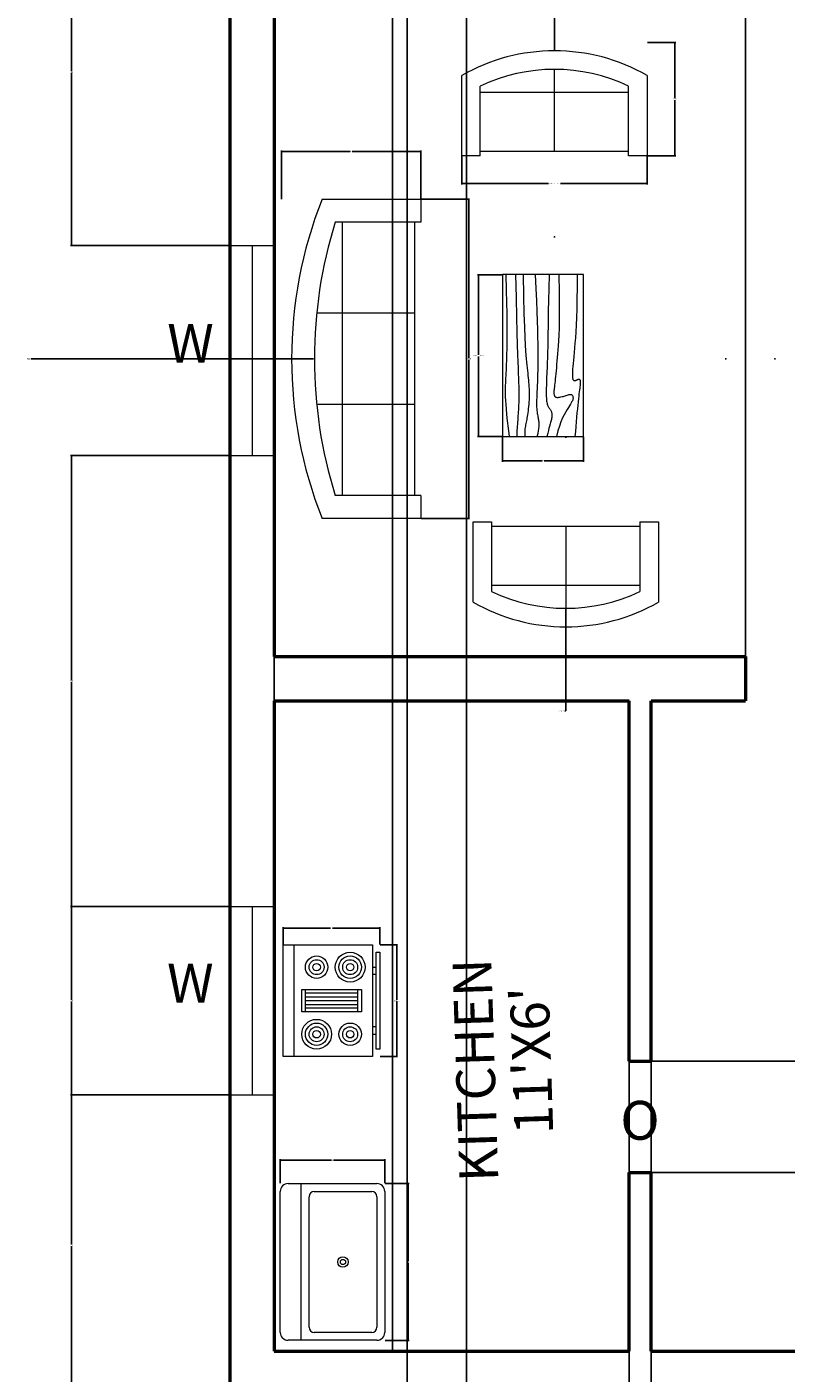
# Model space of a CAD drawing. Units: feet. Extents: x 1657 to 2001, y 1678 to 2367.
# Tile 2 of 4: x 1657 to 1811, y 1847 to 2120. Entities that reach past the tile are written whole.
import ezdxf

# ---------------------------------------------------------------- set-up
doc = ezdxf.new("R2010")
doc.units = ezdxf.units.FT
for name, color, linetype, lineweight in [('A-ANNO-DIMS', 2, 'Continuous', 18), ('A-ANNO-TEXT', 7, 'Continuous', 18), ('A-AREA-IDEN', 7, 'Continuous', 25), ('A-EQPM', 9, 'Continuous', 18), ('A-FLOR-CASE', 8, 'Continuous', 25), ('A-FLOR-FIXT', 8, 'Continuous', 18), ('A-FURN', 8, 'Continuous', 18), ('A-GLAZ', 4, 'Continuous', 18), ('A-WALL', 7, 'Continuous', 50)]:
    doc.layers.add(name, color=color, linetype=linetype, lineweight=lineweight)
doc.styles.get("Standard").update_dxf_attribs({"font": 'arial.ttf'})
doc.dimstyles.get("Standard").update_dxf_attribs({"dimtxt": 0.18, "dimasz": 0.18, "dimexe": 0.18, "dimexo": 0.0625, "dimgap": 0.09, "dimtad": 0, "dimtih": 1, "dimtoh": 1, "dimdec": 4, "dimzin": 0, "dimdsep": 46, "dimtxsty": 'Standard', "dimcen": 0.09, "dimadec": 0, "dimazin": 0, "dimtfac": 1, "dimtdec": 4, "dimtofl": 0, "dimtmove": 0, "dimatfit": 3, "dimfxl": 1, "dimtolj": 1, "dimtzin": 0, "dimarcsym": 0})

# ---------------------------------------------------------------- blocks, each defined once
blk = doc.blocks.new('Sofa - Roundback 7 ft.')
for p, q in [((-12.00002, -32.4421), (-12.00003, -6.5971)), ((11.99997, -32.4421), (11.99998, -6.5971)), ((-36.000027, -34), (-36.000027, -11.4696)), ((-35.999844, -13.3819), (35.9998, -13.3819)), ((35.99998, -34), (35.99998, -11.4696)), ((-36.000027, -32.4421), (35.99998, -32.4421))]:
    blk.add_line(p, q)
for points in [[(-36.000027, -34), (-42.000027, -34), (-42.000027, -8)], [(41.99998, -8), (41.99998, -34), (35.99998, -34)]]:
    blk.add_lwpolyline(points)
for centre, radius, start, end in [((0, -114.25), 114.25, 68.43141, 111.5686), ((-0.00001, -127.1968), 121.1968, 72.72033, 107.2797)]:
    blk.add_arc(centre, radius, start, end)
blk = doc.blocks.new('Sofa - Roundback Loveseat 5 ft.')
for p, q in [((0, -32.44198), (0, -5.99998)), ((-24, -33.99998), (-24, -11.46958)), ((24.00004, -33.99998), (24.00004, -11.46958)), ((-23.9998, -13.38178), (23.99986, -13.38178)), ((-24, -32.44198), (24.00004, -32.44198))]:
    blk.add_line(p, q)
for points in [[(-24, -33.99998), (-30, -33.99998), (-30, -7.99998)], [(30.00004, -7.99998), (30.00004, -33.99998), (24.00004, -33.99998)]]:
    blk.add_lwpolyline(points)
for centre, radius, start, end in [((0, -60.24998), 60.24998, 60.13715, 119.8628), ((0, -61.38438), 55.38444, 64.32083, 115.6792)]:
    blk.add_arc(centre, radius, start, end)
blk = doc.blocks.new('Table - Rectangular Woodgrain 60 x 30 in.')
for p, q in [((0, 0), (0, -30)), ((60, 0), (0, 0)), ((60, -30), (60, 0)), ((0, -30), (60, -30))]:
    blk.add_line(p, q)
for points in [[(0, -2.4), (4.8155, -2.418), (9.0302, -2.4688), (12.709, -2.5477), (15.9167, -2.65), (18.7181, -2.7711), (21.1781, -2.9063), (23.3616, -3.0508), (25.3333, -3.2), (27.1477, -3.3495), (28.8172, -3.4958), (30.3437, -3.636), (31.7291, -3.7667), (32.9756, -3.8849), (34.0849, -3.9875), (35.059, -4.0714), (35.9, -4.1334), (36.6114, -4.1711), (37.2041, -4.1854), (37.6906, -4.1779), (38.0833, -4.15), (38.3948, -4.1034), (38.6375, -4.0396), (38.8239, -3.9602), (38.9666, -3.8667), (39.0764, -3.7608), (39.1573, -3.6448), (39.2116, -3.521), (39.2416, -3.3917), (39.2498, -3.2593), (39.2385, -3.1261), (39.21, -2.9944), (39.1666, -2.8667), (39.111, -2.7447), (39.0468, -2.6281), (38.978, -2.5163), (38.9083, -2.4083), (38.8418, -2.3035), (38.7823, -2.201), (38.7337, -2.1001), (38.7, -2), (38.6844, -1.9003), (38.6875, -1.8021), (38.7094, -1.707), (38.75, -1.6167), (38.8094, -1.5326), (38.8875, -1.4563), (38.9844, -1.3893), (39.1, -1.3333), (39.2351, -1.2896), (39.3937, -1.2583), (39.5804, -1.2396), (39.8, -1.2333), (40.057, -1.2396), (40.3562, -1.2583), (40.7023, -1.2896), (41.1, -1.3333), (41.5547, -1.3895), (42.0755, -1.4573), (42.6721, -1.5361), (43.3542, -1.625), (44.1316, -1.7233), (45.014, -1.8302), (46.0114, -1.9449), (47.1333, -2.0667), (48.3862, -2.1947), (49.7625, -2.3281), (51.2513, -2.4663), (52.8416, -2.6083), (54.5226, -2.7535), (56.2833, -2.9011), (58.1127, -3.0501), (60, -3.2)], [(0, -9.2), (6.5759, -9.0858), (11.9385, -9.0365), (16.2527, -9.0418), (19.6833, -9.0917), (22.3952, -9.1759), (24.5531, -9.2844), (26.322, -9.4069), (27.8666, -9.5333), (29.3241, -9.6553), (30.7203, -9.7719), (32.0532, -9.8837), (33.3208, -9.9917), (34.5213, -10.0965), (35.6526, -10.199), (36.7128, -10.2999), (37.7, -10.4), (38.6129, -10.4996), (39.4531, -10.5969), (40.223, -10.6895), (40.925, -10.775), (41.5613, -10.8512), (42.1344, -10.9156), (42.6465, -10.966), (43.1, -11), (43.4976, -11.0158), (43.8437, -11.0136), (44.143, -10.9942), (44.4, -10.9583), (44.6195, -10.9069), (44.8062, -10.8406), (44.9648, -10.7603), (45.1, -10.6667), (45.2155, -10.5598), (45.3114, -10.4365), (45.3871, -10.2929), (45.4416, -10.125), (45.4743, -9.929), (45.4844, -9.7011), (45.4709, -9.4371), (45.4333, -9.1333), (45.3716, -8.7883), (45.2896, -8.4104), (45.1919, -8.0107), (45.0833, -7.6), (44.9685, -7.1893), (44.8521, -6.7896), (44.7388, -6.4117), (44.6333, -6.0667), (44.54, -5.7628), (44.4614, -5.4979), (44.4001, -5.2675), (44.3583, -5.0667), (44.3384, -4.8909), (44.3427, -4.7354), (44.3736, -4.5956), (44.4333, -4.4667), (44.5236, -4.3453), (44.6427, -4.2333), (44.7884, -4.1339), (44.9583, -4.05), (45.1501, -3.9849), (45.3614, -3.9417), (45.59, -3.9234), (45.8333, -3.9333), (46.0915, -3.9749), (46.3734, -4.0531), (46.6906, -4.1736), (47.0542, -4.3417), (47.4756, -4.5629), (47.9661, -4.8427), (48.5372, -5.1866), (49.2, -5.6), (49.9676, -6.0844), (50.8594, -6.625), (51.8965, -7.2031), (53.1, -7.8), (54.491, -8.3969), (56.0906, -8.975), (57.9199, -9.5156), (60, -10)], [(0, -12.8), (5.1847, -12.9322), (9.6213, -13.0323), (13.3963, -13.1059), (16.5958, -13.1583), (19.3063, -13.1952), (21.614, -13.2219), (23.6054, -13.2439), (25.3666, -13.2667), (26.9728, -13.2947), (28.4531, -13.3281), (29.8256, -13.3663), (31.1083, -13.4083), (32.3191, -13.4535), (33.476, -13.501), (34.597, -13.5501), (35.7, -13.6), (36.7984, -13.6497), (37.8875, -13.6979), (38.9578, -13.743), (40, -13.7833), (41.0047, -13.8174), (41.9625, -13.8438), (42.864, -13.8607), (43.7, -13.8667), (44.4631, -13.8604), (45.1552, -13.8417), (45.7801, -13.8104), (46.3416, -13.7667), (46.8439, -13.7104), (47.2906, -13.6417), (47.6858, -13.5604), (48.0333, -13.4667), (48.3375, -13.3608), (48.6042, -13.2448), (48.8396, -13.121), (49.05, -12.9917), (49.2417, -12.8593), (49.4208, -12.7261), (49.5937, -12.5944), (49.7667, -12.4667), (49.9452, -12.3451), (50.1323, -12.2313), (50.3303, -12.1268), (50.5416, -12.0333), (50.7686, -11.9524), (51.0135, -11.8854), (51.2788, -11.8341), (51.5666, -11.8), (51.8785, -11.7843), (52.2116, -11.7865), (52.562, -11.8059), (52.926, -11.8417), (53.2998, -11.8931), (53.6795, -11.9594), (54.0614, -12.0397), (54.4416, -12.1333), (54.8223, -12.2401), (55.2293, -12.3625), (55.6942, -12.5037), (56.2489, -12.6667), (56.9251, -12.8547), (57.7545, -13.0708), (58.7689, -13.3182), (60, -13.6)], [(0, -18), (5.124, -17.7273), (9.6609, -17.5057), (13.6705, -17.3303), (17.2125, -17.1958), (20.3467, -17.0973), (23.1328, -17.0297), (25.6307, -16.9878), (27.9, -16.9667), (29.9928, -16.9617), (31.9302, -16.9703), (33.7254, -16.9907), (35.3917, -17.0208), (36.9423, -17.0588), (38.3906, -17.1026), (39.7499, -17.1503), (41.0333, -17.2), (42.2519, -17.2496), (43.4073, -17.2969), (44.4986, -17.3395), (45.525, -17.375), (46.4858, -17.4012), (47.3802, -17.4156), (48.2074, -17.416), (48.9667, -17.4), (49.6583, -17.3662), (50.2872, -17.3167), (50.8595, -17.2547), (51.3812, -17.1833), (51.8584, -17.1057), (52.2971, -17.025), (52.7034, -16.9443), (53.0833, -16.8667), (53.443, -16.7951), (53.789, -16.7313), (54.128, -16.6768), (54.4666, -16.6334), (54.8115, -16.6024), (55.1693, -16.5854), (55.5465, -16.5841), (55.95, -16.6), (56.3828, -16.6337), (56.8346, -16.6823), (57.2915, -16.7418), (57.7396, -16.8084), (58.165, -16.878), (58.5539, -16.9469), (58.8924, -17.0111), (59.1666, -17.0667), (59.3679, -17.1107), (59.5078, -17.1438), (59.6032, -17.1675), (59.6708, -17.1833), (59.7275, -17.193), (59.7901, -17.1979), (59.8753, -17.1998), (60, -17.2)], [(0, -22.4), (8.0098, -22.2501), (14.4094, -22.1011), (19.4168, -21.9535), (23.25, -21.8083), (26.1269, -21.6663), (28.2656, -21.5281), (29.884, -21.3947), (31.2, -21.2667), (32.3967, -21.1448), (33.5172, -21.0292), (34.5697, -20.9198), (35.5625, -20.8167), (36.5037, -20.7198), (37.4015, -20.6292), (38.2642, -20.5448), (39.1, -20.4667), (39.9164, -20.3951), (40.7187, -20.3313), (41.5117, -20.2768), (42.3, -20.2333), (43.0883, -20.2024), (43.8812, -20.1854), (44.6836, -20.1841), (45.5, -20.2), (46.3328, -20.234), (47.1747, -20.2844), (48.0163, -20.3488), (48.8479, -20.425), (49.66, -20.5106), (50.4429, -20.6031), (51.1872, -20.7004), (51.8833, -20.8), (52.5246, -20.8999), (53.1166, -20.9995), (53.6681, -21.0983), (54.1875, -21.1958), (54.6834, -21.2919), (55.1646, -21.3859), (55.6394, -21.4777), (56.1167, -21.5667), (56.6028, -21.6515), (57.0961, -21.7266), (57.5929, -21.7852), (58.0896, -21.8208), (58.5823, -21.8268), (59.0674, -21.7964), (59.5412, -21.723), (60, -21.6)], [(0, -25.2), (8.6355, -25.0504), (15.7026, -24.9031), (21.4049, -24.7606), (25.9458, -24.625), (29.529, -24.4988), (32.3578, -24.3844), (34.6359, -24.284), (36.5667, -24.2), (38.3213, -24.1341), (39.9417, -24.0854), (41.437, -24.0523), (42.8167, -24.0333), (44.0901, -24.0268), (45.2667, -24.0313), (46.3557, -24.0451), (47.3667, -24.0667), (48.309, -24.0947), (49.1928, -24.1287), (50.0284, -24.168), (50.826, -24.2125), (51.5959, -24.2617), (52.3483, -24.3151), (53.0935, -24.3725), (53.8417, -24.4334), (54.6009, -24.497), (55.3699, -24.561), (56.1454, -24.6226), (56.9239, -24.6792), (57.7021, -24.7279), (58.4764, -24.7662), (59.2435, -24.7911), (60, -24.8)], [(0, -28.8), (5.6867, -28.6681), (10.45, -28.5698), (14.407, -28.5012), (17.675, -28.4584), (20.3711, -28.4374), (22.6125, -28.4344), (24.5164, -28.4455), (26.2, -28.4667), (27.762, -28.4947), (29.2276, -28.5281), (30.6033, -28.5663), (31.8958, -28.6084), (33.1118, -28.6535), (34.2578, -28.7011), (35.3405, -28.7501), (36.3666, -28.8), (37.3443, -28.8497), (38.288, -28.8974), (39.2137, -28.9412), (40.1375, -28.9792), (41.0753, -29.0093), (42.0432, -29.0297), (43.0572, -29.0384), (44.1333, -29.0333), (45.2936, -29.0114), (46.5843, -28.9641), (48.0579, -28.8816), (49.7666, -28.7542), (51.7629, -28.5721), (54.0989, -28.3255), (56.8272, -28.0048), (60, -27.6)]]:
    blk.add_lwpolyline(points)
blk = doc.blocks.new('Range-Oven - 30 in top')
for p, q in [((0, -3), (30, -3)), ((12, -6), (18, -6)), ((13, -20), (13, -6)), ((14, -6), (14, -20)), ((15, -20), (15, -6)), ((16, -6), (16, -20)), ((17, -20), (17, -6)), ((18, -20), (12, -20)), ((6, -24), (6, -25)), ((8, -25), (8, -24)), ((22, -25), (22, -24)), ((24, -24), (24, -25))]:
    blk.add_line(p, q)
for points in [[(0, -24), (0, 0), (30, 0), (30, -24)], [(12, -21), (12, -5), (18, -5), (18, -21)], [(2, -26), (2, -25), (28, -25), (28, -26)]]:
    blk.add_lwpolyline(points, close=True)
for centre, radius in [((6, -9), 4), ((6, -9), 3), ((6, -9), 2), ((24, -9), 3), ((24, -9), 2), ((6, -9), 1), ((24, -9), 1), ((24, -18), 4), ((6, -18), 3), ((6, -18), 2), ((6, -18), 1), ((24, -18), 3), ((24, -18), 2), ((24, -18), 1)]:
    blk.add_circle(centre, radius)
blk = doc.blocks.new('Sink-single - 30 in top')
blk.add_line((-15, -3.999996), (15, -3.999996))
for points in [[(-13.5, 0), (13.5, 0)], [(-15, -18.499996), (-15, -1.5)], [(15, -1.5), (15, -18.499996)], [(-13.5, -17.499996), (-13.5, -6.499996)], [(-12.5, -5.499996), (12.5, -5.499996)], [(13.5, -6.499996), (13.5, -17.499996)], [(13.5, -19.999996), (-13.5, -19.999996)], [(12.5, -18.499996), (-12.5, -18.499996)]]:
    blk.add_lwpolyline(points)
for radius in [1, 0.5]:
    blk.add_circle((0, -11.999996), radius)
for centre, radius, start, end in [((-13.5, -1.5), 1.5, 90, 180), ((13.5, -1.5), 1.5, 0, 90), ((-12.5, -6.499996), 1, 90, 180), ((12.5, -6.499996), 1, 0, 90), ((-12.5, -17.499996), 1, 180, 270), ((12.5, -17.499996), 1, 270, 0), ((-13.5, -18.499996), 1.5, 180, 270), ((13.5, -18.499996), 1.5, 270, 0)]:
    blk.add_arc(centre, radius, start, end)
blk = doc.blocks.new('WIN-HALL')
for p, q in [((0, 42.59), (9, 42.59)), ((4.5, 42.59), (4.5, 0)), ((0, 0), (9, 0))]:
    blk.add_line(p, q)
blk = doc.blocks.new('*D16')
at = {"layer": 'A-ANNO-DIMS', "color": 0, "lineweight": -2, "transparency": 16777216}
for p, q in [((1745.34, 2093.87), (1745.34, 2088.11)), ((1782.96, 2093.87), (1782.96, 2088.11)), ((1745.52, 2088.29), (1762.93, 2088.29)), ((1782.78, 2088.29), (1765.37, 2088.29))]:
    blk.add_line(p, q, dxfattribs=at)
at = {"layer": 'A-ANNO-DIMS', "color": 0, "transparency": 16777216}
for points in [[(1745.52, 2088.32), (1745.52, 2088.26), (1745.34, 2088.29)], [(1782.78, 2088.32), (1782.78, 2088.26), (1782.96, 2088.29)]]:
    blk.add_solid(points, dxfattribs=at)
at = {"layer": 'Defpoints', "color": 0, "transparency": 16777216}
for p in [(1745.34, 2093.93), (1782.96, 2093.93), (1782.96, 2088.29)]:
    blk.add_point(p, dxfattribs=at)
at = {"layer": 'A-ANNO-DIMS', "color": 0, "transparency": 16777216, "insert": (1764.15, 2088.29), "char_height": 0.18, "attachment_point": 5}
blk.add_mtext('\\A1;LOVESEAT 38 TYP.', dxfattribs=at)
blk = doc.blocks.new('*D17')
at = {"layer": 'A-ANNO-DIMS', "color": 0, "lineweight": -2, "transparency": 16777216}
for p, q in [((1783.02, 2116.92), (1788.78, 2116.92)), ((1788.6, 2116.74), (1788.6, 2105.61)), ((1788.6, 2094.11), (1788.6, 2105.24)), ((1783.02, 2093.93), (1788.78, 2093.93))]:
    blk.add_line(p, q, dxfattribs=at)
at = {"layer": 'A-ANNO-DIMS', "color": 0, "transparency": 16777216}
for points in [[(1788.57, 2116.74), (1788.63, 2116.74), (1788.6, 2116.92)], [(1788.57, 2094.11), (1788.63, 2094.11), (1788.6, 2093.93)]]:
    blk.add_solid(points, dxfattribs=at)
at = {"layer": 'Defpoints', "color": 0, "transparency": 16777216}
for p in [(1782.96, 2116.92), (1788.6, 2116.92), (1782.96, 2093.93)]:
    blk.add_point(p, dxfattribs=at)
at = {"layer": 'A-ANNO-DIMS', "color": 0, "transparency": 16777216, "insert": (1788.6, 2105.42), "char_height": 0.18, "attachment_point": 5}
blk.add_mtext('\\A1;23 TYP.', dxfattribs=at)
blk = doc.blocks.new('*D18')
at = {"layer": 'A-ANNO-DIMS', "color": 0, "lineweight": -2, "transparency": 16777216}
for p, q in [((1737.09, 2085.11), (1746.92, 2085.11)), ((1746.74, 2084.93), (1746.74, 2052.91)), ((1746.74, 2020.53), (1746.74, 2052.55)), ((1737.09, 2020.35), (1746.92, 2020.35))]:
    blk.add_line(p, q, dxfattribs=at)
at = {"layer": 'A-ANNO-DIMS', "color": 0, "transparency": 16777216}
for points in [[(1746.71, 2084.93), (1746.77, 2084.93), (1746.74, 2085.11)], [(1746.71, 2020.53), (1746.77, 2020.53), (1746.74, 2020.35)]]:
    blk.add_solid(points, dxfattribs=at)
at = {"layer": 'Defpoints', "color": 0, "transparency": 16777216}
for p in [(1737.03, 2085.11), (1746.74, 2085.11), (1737.03, 2020.35)]:
    blk.add_point(p, dxfattribs=at)
at = {"layer": 'A-ANNO-DIMS', "color": 0, "transparency": 16777216, "insert": (1746.74, 2052.73), "char_height": 0.18, "attachment_point": 5}
blk.add_mtext('\\A1;SOFA 65', dxfattribs=at)
blk = doc.blocks.new('*D19')
at = {"layer": 'A-ANNO-DIMS', "color": 0, "lineweight": -2, "transparency": 16777216}
for p, q in [((1708.76, 2085.17), (1708.76, 2095.01)), ((1708.94, 2094.83), (1722.67, 2094.83)), ((1736.85, 2094.83), (1723.11, 2094.83)), ((1737.03, 2085.17), (1737.03, 2095.01))]:
    blk.add_line(p, q, dxfattribs=at)
at = {"layer": 'A-ANNO-DIMS', "color": 0, "transparency": 16777216}
for points in [[(1708.94, 2094.86), (1708.94, 2094.8), (1708.76, 2094.83)], [(1736.85, 2094.86), (1736.85, 2094.8), (1737.03, 2094.83)]]:
    blk.add_solid(points, dxfattribs=at)
at = {"layer": 'Defpoints', "color": 0, "transparency": 16777216}
for p in [(1708.76, 2094.83), (1708.76, 2085.11), (1737.03, 2085.11)]:
    blk.add_point(p, dxfattribs=at)
at = {"layer": 'A-ANNO-DIMS', "color": 0, "transparency": 16777216, "insert": (1722.89, 2094.83), "char_height": 0.18, "attachment_point": 5}
blk.add_mtext('\\A1;28', dxfattribs=at)
blk = doc.blocks.new('*D20')
at = {"layer": 'A-ANNO-DIMS', "color": 0, "lineweight": -2, "transparency": 16777216}
for p, q in [((1753.57, 2069.81), (1748.52, 2069.81)), ((1748.7, 2069.63), (1748.7, 2053.56)), ((1748.7, 2037.13), (1748.7, 2053.2)), ((1753.57, 2036.95), (1748.52, 2036.95))]:
    blk.add_line(p, q, dxfattribs=at)
at = {"layer": 'A-ANNO-DIMS', "color": 0, "transparency": 16777216}
for points in [[(1748.67, 2069.63), (1748.73, 2069.63), (1748.7, 2069.81)], [(1748.67, 2037.13), (1748.73, 2037.13), (1748.7, 2036.95)]]:
    blk.add_solid(points, dxfattribs=at)
at = {"layer": 'Defpoints', "color": 0, "transparency": 16777216}
for p in [(1753.63, 2069.81), (1748.7, 2036.95), (1753.63, 2036.95)]:
    blk.add_point(p, dxfattribs=at)
at = {"layer": 'A-ANNO-DIMS', "color": 0, "transparency": 16777216, "insert": (1748.7, 2053.38), "char_height": 0.18, "attachment_point": 5}
blk.add_mtext('\\A1;COFFEE TABLE 33', dxfattribs=at)
blk = doc.blocks.new('*D21')
at = {"layer": 'A-ANNO-DIMS', "color": 0, "lineweight": -2, "transparency": 16777216}
for p, q in [((1753.63, 2036.88), (1753.63, 2031.84)), ((1770.07, 2036.88), (1770.07, 2031.84)), ((1753.81, 2032.02), (1761.64, 2032.02)), ((1769.89, 2032.02), (1762.06, 2032.02))]:
    blk.add_line(p, q, dxfattribs=at)
at = {"layer": 'A-ANNO-DIMS', "color": 0, "transparency": 16777216}
for points in [[(1753.81, 2032.05), (1753.81, 2031.99), (1753.63, 2032.02)], [(1769.89, 2032.05), (1769.89, 2031.99), (1770.07, 2032.02)]]:
    blk.add_solid(points, dxfattribs=at)
at = {"layer": 'Defpoints', "color": 0, "transparency": 16777216}
for p in [(1753.63, 2036.95), (1770.07, 2036.95), (1770.07, 2032.02)]:
    blk.add_point(p, dxfattribs=at)
at = {"layer": 'A-ANNO-DIMS', "color": 0, "transparency": 16777216, "insert": (1761.85, 2032.02), "char_height": 0.18, "attachment_point": 5}
blk.add_mtext('\\A1;16', dxfattribs=at)
blk = doc.blocks.new('*D24')
at = {"layer": 'A-ANNO-DIMS', "color": 0, "lineweight": -2, "transparency": 16777216}
for p, q in [((1728.8, 1933.8), (1732.33, 1933.8)), ((1732.15, 1933.62), (1732.15, 1922.64)), ((1732.15, 1911.29), (1732.15, 1922.27)), ((1728.8, 1911.11), (1732.33, 1911.11))]:
    blk.add_line(p, q, dxfattribs=at)
at = {"layer": 'A-ANNO-DIMS', "color": 0, "transparency": 16777216}
for points in [[(1732.12, 1933.62), (1732.18, 1933.62), (1732.15, 1933.8)], [(1732.12, 1911.29), (1732.18, 1911.29), (1732.15, 1911.11)]]:
    blk.add_solid(points, dxfattribs=at)
at = {"layer": 'Defpoints', "color": 0, "transparency": 16777216}
for p in [(1728.74, 1933.8), (1732.15, 1933.8), (1728.74, 1911.11)]:
    blk.add_point(p, dxfattribs=at)
at = {"layer": 'A-ANNO-DIMS', "color": 0, "transparency": 16777216, "insert": (1732.15, 1922.45), "char_height": 0.18, "attachment_point": 5}
blk.add_mtext('\\A1;RANGE 23', dxfattribs=at)
blk = doc.blocks.new('*D25')
at = {"layer": 'A-ANNO-DIMS', "color": 0, "lineweight": -2, "transparency": 16777216}
for p, q in [((1709.07, 1933.86), (1709.07, 1937.38)), ((1709.25, 1937.2), (1718.69, 1937.2)), ((1728.56, 1937.2), (1719.13, 1937.2)), ((1728.74, 1933.86), (1728.74, 1937.38))]:
    blk.add_line(p, q, dxfattribs=at)
at = {"layer": 'A-ANNO-DIMS', "color": 0, "transparency": 16777216}
for points in [[(1709.25, 1937.23), (1709.25, 1937.17), (1709.07, 1937.2)], [(1728.56, 1937.23), (1728.56, 1937.17), (1728.74, 1937.2)]]:
    blk.add_solid(points, dxfattribs=at)
at = {"layer": 'Defpoints', "color": 0, "transparency": 16777216}
for p in [(1709.07, 1937.2), (1709.07, 1933.8), (1728.74, 1933.8)]:
    blk.add_point(p, dxfattribs=at)
at = {"layer": 'A-ANNO-DIMS', "color": 0, "transparency": 16777216, "insert": (1718.91, 1937.2), "char_height": 0.18, "attachment_point": 5}
blk.add_mtext('\\A1;20', dxfattribs=at)
blk = doc.blocks.new('*D26')
at = {"layer": 'A-ANNO-DIMS', "color": 0, "lineweight": -2, "transparency": 16777216}
for p, q in [((1729.77, 1885.33), (1734.66, 1885.33)), ((1734.48, 1885.15), (1734.48, 1869.61)), ((1734.48, 1853.7), (1734.48, 1869.24)), ((1729.77, 1853.52), (1734.66, 1853.52))]:
    blk.add_line(p, q, dxfattribs=at)
at = {"layer": 'A-ANNO-DIMS', "color": 0, "transparency": 16777216}
for points in [[(1734.45, 1885.15), (1734.51, 1885.15), (1734.48, 1885.33)], [(1734.45, 1853.7), (1734.51, 1853.7), (1734.48, 1853.52)]]:
    blk.add_solid(points, dxfattribs=at)
at = {"layer": 'Defpoints', "color": 0, "transparency": 16777216}
for p in [(1729.71, 1885.33), (1734.48, 1885.33), (1729.71, 1853.52)]:
    blk.add_point(p, dxfattribs=at)
at = {"layer": 'A-ANNO-DIMS', "color": 0, "transparency": 16777216, "insert": (1734.48, 1869.42), "char_height": 0.18, "attachment_point": 5}
blk.add_mtext('\\A1;SINK 32', dxfattribs=at)
blk = doc.blocks.new('*D27')
at = {"layer": 'A-ANNO-DIMS', "color": 0, "lineweight": -2, "transparency": 16777216}
for p, q in [((1708.51, 1885.39), (1708.51, 1890.28)), ((1708.69, 1890.1), (1718.91, 1890.1)), ((1729.53, 1890.1), (1719.31, 1890.1)), ((1729.71, 1885.39), (1729.71, 1890.28))]:
    blk.add_line(p, q, dxfattribs=at)
at = {"layer": 'A-ANNO-DIMS', "color": 0, "transparency": 16777216}
for points in [[(1708.69, 1890.13), (1708.69, 1890.07), (1708.51, 1890.1)], [(1729.53, 1890.13), (1729.53, 1890.07), (1729.71, 1890.1)]]:
    blk.add_solid(points, dxfattribs=at)
at = {"layer": 'Defpoints', "color": 0, "transparency": 16777216}
for p in [(1708.51, 1890.1), (1708.51, 1885.33), (1729.71, 1885.33)]:
    blk.add_point(p, dxfattribs=at)
at = {"layer": 'A-ANNO-DIMS', "color": 0, "transparency": 16777216, "insert": (1719.11, 1890.1), "char_height": 0.18, "attachment_point": 5}
blk.add_mtext('\\A1;21', dxfattribs=at)
blk = doc.blocks.new('*D37')
at = {"layer": 'A-ANNO-DIMS', "color": 0, "lineweight": -2, "transparency": 16777216}
for p, q in [((1734.28, 1770.36), (1734.28, 2366.63)), ((1734.46, 2366.45), (1740.08, 2366.45)), ((1746.1, 2366.45), (1740.49, 2366.45)), ((1746.28, 1770.36), (1746.28, 2366.63))]:
    blk.add_line(p, q, dxfattribs=at)
at = {"layer": 'A-ANNO-DIMS', "color": 0, "transparency": 16777216}
for points in [[(1734.46, 2366.48), (1734.46, 2366.42), (1734.28, 2366.45)], [(1746.1, 2366.48), (1746.1, 2366.42), (1746.28, 2366.45)]]:
    blk.add_solid(points, dxfattribs=at)
at = {"layer": 'Defpoints', "color": 0, "transparency": 16777216}
for p in [(1746.28, 2366.45), (1734.28, 1770.3), (1746.28, 1770.3)]:
    blk.add_point(p, dxfattribs=at)
at = {"layer": 'A-ANNO-DIMS', "color": 0, "transparency": 16777216, "insert": (1740.28, 2366.45), "char_height": 0.18, "attachment_point": 5}
blk.add_mtext('\\A1;12', dxfattribs=at)
blk = doc.blocks.new('*D38')
at = {"layer": 'A-ANNO-DIMS', "color": 0, "lineweight": -2, "transparency": 16777216}
for p, q in [((1698.28, 1770.36), (1698.28, 2366.63)), ((1698.46, 2366.45), (1716.07, 2366.45)), ((1734.1, 2366.45), (1716.5, 2366.45)), ((1734.28, 1770.36), (1734.28, 2366.63))]:
    blk.add_line(p, q, dxfattribs=at)
at = {"layer": 'A-ANNO-DIMS', "color": 0, "transparency": 16777216}
for points in [[(1698.46, 2366.48), (1698.46, 2366.42), (1698.28, 2366.45)], [(1734.1, 2366.48), (1734.1, 2366.42), (1734.28, 2366.45)]]:
    blk.add_solid(points, dxfattribs=at)
at = {"layer": 'Defpoints', "color": 0, "transparency": 16777216}
for p in [(1734.28, 2366.45), (1698.28, 1770.3), (1734.28, 1770.3)]:
    blk.add_point(p, dxfattribs=at)
at = {"layer": 'A-ANNO-DIMS', "color": 0, "transparency": 16777216, "insert": (1716.28, 2366.45), "char_height": 0.18, "attachment_point": 5}
blk.add_mtext('\\A1;36', dxfattribs=at)
blk = doc.blocks.new('*D43')
at = {"layer": 'A-ANNO-DIMS', "color": 0, "lineweight": -2, "transparency": 16777216}
for p, q in [((1698.22, 1903.34), (1665.95, 1903.34)), ((1666.13, 1903.16), (1666.13, 1873)), ((1666.13, 1842.48), (1666.13, 1872.64)), ((1698.22, 1842.3), (1665.95, 1842.3))]:
    blk.add_line(p, q, dxfattribs=at)
at = {"layer": 'A-ANNO-DIMS', "color": 0, "transparency": 16777216}
for points in [[(1666.1, 1903.16), (1666.16, 1903.16), (1666.13, 1903.34)], [(1666.1, 1842.48), (1666.16, 1842.48), (1666.13, 1842.3)]]:
    blk.add_solid(points, dxfattribs=at)
at = {"layer": 'Defpoints', "color": 0, "transparency": 16777216}
for p in [(1666.13, 1903.34), (1698.28, 1903.34), (1698.28, 1842.3)]:
    blk.add_point(p, dxfattribs=at)
at = {"layer": 'A-ANNO-DIMS', "color": 0, "transparency": 16777216, "insert": (1666.13, 1872.82), "char_height": 0.18, "attachment_point": 5}
blk.add_mtext('\\A1;61.04', dxfattribs=at)
blk = doc.blocks.new('*D44')
at = {"layer": 'A-ANNO-DIMS', "color": 0, "lineweight": -2, "transparency": 16777216}
for p, q in [((1698.22, 1941.58), (1665.95, 1941.58)), ((1666.13, 1941.4), (1666.13, 1922.64)), ((1666.13, 1903.52), (1666.13, 1922.28)), ((1698.22, 1903.34), (1665.95, 1903.34))]:
    blk.add_line(p, q, dxfattribs=at)
at = {"layer": 'A-ANNO-DIMS', "color": 0, "transparency": 16777216}
for points in [[(1666.1, 1941.4), (1666.16, 1941.4), (1666.13, 1941.58)], [(1666.1, 1903.52), (1666.16, 1903.52), (1666.13, 1903.34)]]:
    blk.add_solid(points, dxfattribs=at)
at = {"layer": 'Defpoints', "color": 0, "transparency": 16777216}
for p in [(1666.13, 1941.58), (1698.28, 1941.58), (1698.28, 1903.34)]:
    blk.add_point(p, dxfattribs=at)
at = {"layer": 'A-ANNO-DIMS', "color": 0, "transparency": 16777216, "insert": (1666.13, 1922.46), "char_height": 0.18, "attachment_point": 5}
blk.add_mtext('\\A1;38.24', dxfattribs=at)
blk = doc.blocks.new('*D45')
at = {"layer": 'A-ANNO-DIMS', "color": 0, "lineweight": -2, "transparency": 16777216}
for p, q in [((1698.22, 2033.14), (1665.95, 2033.14)), ((1666.13, 2032.96), (1666.13, 1987.54)), ((1666.13, 1941.76), (1666.13, 1987.18)), ((1698.22, 1941.58), (1665.95, 1941.58))]:
    blk.add_line(p, q, dxfattribs=at)
at = {"layer": 'A-ANNO-DIMS', "color": 0, "transparency": 16777216}
for points in [[(1666.1, 2032.96), (1666.16, 2032.96), (1666.13, 2033.14)], [(1666.1, 1941.76), (1666.16, 1941.76), (1666.13, 1941.58)]]:
    blk.add_solid(points, dxfattribs=at)
at = {"layer": 'Defpoints', "color": 0, "transparency": 16777216}
for p in [(1666.13, 2033.14), (1698.28, 2033.14), (1698.28, 1941.58)]:
    blk.add_point(p, dxfattribs=at)
at = {"layer": 'A-ANNO-DIMS', "color": 0, "transparency": 16777216, "insert": (1666.13, 1987.36), "char_height": 0.18, "attachment_point": 5}
blk.add_mtext('\\A1;91.57', dxfattribs=at)
blk = doc.blocks.new('*D46')
at = {"layer": 'A-ANNO-DIMS', "color": 0, "lineweight": -2, "transparency": 16777216}
for p, q in [((1698.22, 2146.17), (1665.95, 2146.17)), ((1666.13, 2145.99), (1666.13, 2111.13)), ((1666.13, 2075.91), (1666.13, 2110.77)), ((1698.22, 2075.73), (1665.95, 2075.73))]:
    blk.add_line(p, q, dxfattribs=at)
at = {"layer": 'A-ANNO-DIMS', "color": 0, "transparency": 16777216}
for points in [[(1666.1, 2145.99), (1666.16, 2145.99), (1666.13, 2146.17)], [(1666.1, 2075.91), (1666.16, 2075.91), (1666.13, 2075.73)]]:
    blk.add_solid(points, dxfattribs=at)
at = {"layer": 'Defpoints', "color": 0, "transparency": 16777216}
for p in [(1666.13, 2146.17), (1698.28, 2146.17), (1698.28, 2075.73)]:
    blk.add_point(p, dxfattribs=at)
at = {"layer": 'A-ANNO-DIMS', "color": 0, "transparency": 16777216, "insert": (1666.13, 2110.95), "char_height": 0.18, "attachment_point": 5}
blk.add_mtext('\\A1;70.44', dxfattribs=at)
blk = doc.blocks.new('*D53')
at = {"layer": 'A-ANNO-DIMS', "color": 0, "lineweight": -2, "transparency": 16777216}
for p, q in [((1779.28, 1983.24), (1779.28, 1677.97)), ((1783.78, 1983.24), (1783.78, 1677.97)), ((1779.46, 1678.15), (1781.28, 1678.15)), ((1783.6, 1678.15), (1781.79, 1678.15))]:
    blk.add_line(p, q, dxfattribs=at)
at = {"layer": 'A-ANNO-DIMS', "color": 0, "transparency": 16777216}
for points in [[(1779.46, 1678.18), (1779.46, 1678.12), (1779.28, 1678.15)], [(1783.6, 1678.18), (1783.6, 1678.12), (1783.78, 1678.15)]]:
    blk.add_solid(points, dxfattribs=at)
at = {"layer": 'Defpoints', "color": 0, "transparency": 16777216}
for p in [(1779.28, 1983.3), (1783.78, 1983.3), (1783.78, 1678.15)]:
    blk.add_point(p, dxfattribs=at)
at = {"layer": 'A-ANNO-DIMS', "color": 0, "transparency": 16777216, "insert": (1781.53, 1678.15), "char_height": 0.18, "attachment_point": 5}
blk.add_mtext('\\A1;4.5', dxfattribs=at)
blk = doc.blocks.new('*D54')
at = {"layer": 'A-ANNO-DIMS', "color": 0, "lineweight": -2, "transparency": 16777216}
for p, q in [((1779.35, 1910.16), (2000.61, 1910.16)), ((2000.43, 1909.98), (2000.43, 1899.06)), ((2000.43, 1887.77), (2000.43, 1898.69)), ((1779.35, 1887.59), (2000.61, 1887.59))]:
    blk.add_line(p, q, dxfattribs=at)
at = {"layer": 'A-ANNO-DIMS', "color": 0, "transparency": 16777216}
for points in [[(2000.4, 1909.98), (2000.46, 1909.98), (2000.43, 1910.16)], [(2000.4, 1887.77), (2000.46, 1887.77), (2000.43, 1887.59)]]:
    blk.add_solid(points, dxfattribs=at)
at = {"layer": 'Defpoints', "color": 0, "transparency": 16777216}
for p in [(1779.28, 1910.16), (2000.43, 1910.16), (1779.28, 1887.59)]:
    blk.add_point(p, dxfattribs=at)
at = {"layer": 'A-ANNO-DIMS', "color": 0, "transparency": 16777216, "insert": (2000.43, 1898.88), "char_height": 0.18, "attachment_point": 5}
blk.add_mtext('\\A1;22.577', dxfattribs=at)
blk = doc.blocks.new('*D55')
at = {"layer": 'A-ANNO-DIMS', "color": 0, "lineweight": -2, "transparency": 16777216}
for p, q in [((1707.28, 1851.36), (1707.28, 2366.63)), ((1707.46, 2366.45), (1719.06, 2366.45)), ((1731.1, 2366.45), (1719.5, 2366.45)), ((1731.28, 1851.36), (1731.28, 2366.63))]:
    blk.add_line(p, q, dxfattribs=at)
at = {"layer": 'A-ANNO-DIMS', "color": 0, "transparency": 16777216}
for points in [[(1707.46, 2366.48), (1707.46, 2366.42), (1707.28, 2366.45)], [(1731.1, 2366.48), (1731.1, 2366.42), (1731.28, 2366.45)]]:
    blk.add_solid(points, dxfattribs=at)
at = {"layer": 'Defpoints', "color": 0, "transparency": 16777216}
for p in [(1731.28, 2366.45), (1707.28, 1851.3), (1731.28, 1851.3)]:
    blk.add_point(p, dxfattribs=at)
at = {"layer": 'A-ANNO-DIMS', "color": 0, "transparency": 16777216, "insert": (1719.28, 2366.45), "char_height": 0.18, "attachment_point": 5}
blk.add_mtext('\\A1;24', dxfattribs=at)
blk = doc.blocks.new('*D56')
at = {"layer": 'A-ANNO-DIMS', "color": 0, "lineweight": -2, "transparency": 16777216}
for p, q in [((1802.91, 1992.36), (1802.91, 2366.63)), ((1803.09, 2366.45), (1828.29, 2366.45)), ((1854.28, 2366.45), (1829.08, 2366.45)), ((1854.46, 1992.36), (1854.46, 2366.63))]:
    blk.add_line(p, q, dxfattribs=at)
at = {"layer": 'A-ANNO-DIMS', "color": 0, "transparency": 16777216}
for points in [[(1803.09, 2366.48), (1803.09, 2366.42), (1802.91, 2366.45)], [(1854.28, 2366.48), (1854.28, 2366.42), (1854.46, 2366.45)]]:
    blk.add_solid(points, dxfattribs=at)
at = {"layer": 'Defpoints', "color": 0, "transparency": 16777216}
for p in [(1854.46, 2366.45), (1802.91, 1992.3), (1854.46, 1992.3)]:
    blk.add_point(p, dxfattribs=at)
at = {"layer": 'A-ANNO-DIMS', "color": 0, "transparency": 16777216, "insert": (1828.68, 2366.45), "char_height": 0.18, "attachment_point": 5}
blk.add_mtext('\\A1;51.55', dxfattribs=at)
blk = doc.blocks.new('*D63')
at = {"layer": 'A-ANNO-DIMS', "color": 0, "lineweight": -2, "transparency": 16777216}
for p, q in [((1659.37, 2052.73), (1715.26, 2052.73)), ((1808.79, 2052.73), (1808.97, 2052.73)), ((1808.88, 2052.64), (1808.88, 2052.82))]:
    blk.add_line(p, q, dxfattribs=at)
at = {"layer": 'A-ANNO-DIMS', "color": 0, "transparency": 16777216}
blk.add_solid([(1715.26, 2052.76), (1715.26, 2052.7), (1715.44, 2052.73)], dxfattribs=at)
at = {"layer": 'Defpoints', "color": 0, "transparency": 16777216}
for p in [(1715.44, 2052.73), (1808.88, 2052.73)]:
    blk.add_point(p, dxfattribs=at)
at = {"layer": 'A-ANNO-DIMS', "color": 0, "transparency": 16777216, "insert": (1658.9, 2052.73), "char_height": 0.18, "attachment_point": 5}
blk.add_mtext('\\A1;R93.44', dxfattribs=at)
blk = doc.blocks.new('*D64')
at = {"layer": 'A-ANNO-DIMS', "color": 0, "lineweight": -2, "transparency": 16777216}
for p, q in [((1657.96, 2052.73), (1710.63, 2052.73)), ((1798.81, 2052.73), (1798.99, 2052.73)), ((1798.9, 2052.64), (1798.9, 2052.82))]:
    blk.add_line(p, q, dxfattribs=at)
at = {"layer": 'A-ANNO-DIMS', "color": 0, "transparency": 16777216}
blk.add_solid([(1710.63, 2052.76), (1710.63, 2052.7), (1710.81, 2052.73)], dxfattribs=at)
at = {"layer": 'Defpoints', "color": 0, "transparency": 16777216}
for p in [(1710.81, 2052.73), (1798.9, 2052.73)]:
    blk.add_point(p, dxfattribs=at)
at = {"layer": 'A-ANNO-DIMS', "color": 0, "transparency": 16777216, "insert": (1657.48, 2052.73), "char_height": 0.18, "attachment_point": 5}
blk.add_mtext('\\A1;R88.08', dxfattribs=at)
blk = doc.blocks.new('*D65')
at = {"layer": 'A-ANNO-DIMS', "color": 0, "lineweight": -2, "transparency": 16777216}
for p, q in [((1764.33, 2137.91), (1764.15, 2137.91)), ((1764.15, 2137.91), (1764.15, 2115.43)), ((1764.06, 2077.47), (1764.24, 2077.47)), ((1764.15, 2077.38), (1764.15, 2077.56))]:
    blk.add_line(p, q, dxfattribs=at)
at = {"layer": 'A-ANNO-DIMS', "color": 0, "transparency": 16777216}
blk.add_solid([(1764.12, 2115.43), (1764.18, 2115.43), (1764.15, 2115.25)], dxfattribs=at)
at = {"layer": 'Defpoints', "color": 0, "transparency": 16777216}
for p in [(1764.15, 2115.25), (1764.15, 2077.47)]:
    blk.add_point(p, dxfattribs=at)
at = {"layer": 'A-ANNO-DIMS', "color": 0, "transparency": 16777216, "insert": (1765.07, 2137.91), "char_height": 0.18, "attachment_point": 5}
blk.add_mtext('\\A1;2X R37.776', dxfattribs=at)
blk = doc.blocks.new('*D66')
at = {"layer": 'A-ANNO-DIMS', "color": 0, "lineweight": -2, "transparency": 16777216}
for p, q in [((1766.36, 2036.82), (1766.54, 2036.82)), ((1766.45, 2036.73), (1766.45, 2036.91)), ((1766.45, 1981.26), (1766.45, 2001.92)), ((1766.27, 1981.26), (1766.45, 1981.26))]:
    blk.add_line(p, q, dxfattribs=at)
at = {"layer": 'A-ANNO-DIMS', "color": 0, "transparency": 16777216}
blk.add_solid([(1766.42, 2001.92), (1766.48, 2001.92), (1766.45, 2002.1)], dxfattribs=at)
at = {"layer": 'Defpoints', "color": 0, "transparency": 16777216}
for p in [(1766.45, 2036.82), (1766.45, 2002.1)]:
    blk.add_point(p, dxfattribs=at)
at = {"layer": 'A-ANNO-DIMS', "color": 0, "transparency": 16777216, "insert": (1765.53, 1981.26), "char_height": 0.18, "attachment_point": 5}
blk.add_mtext('\\A1;2X R34.725', dxfattribs=at)

msp = doc.modelspace()

# ---------------------------------------------------------------- linework, layer by layer
at = {"layer": 'A-FLOR-CASE'}
msp.add_line((1731.2848, 1983.2977), (1731.2848, 1851.2977), dxfattribs=at)
at = {"layer": 'A-GLAZ'}
for p, q in [((1698.2848, 1941.5784), (1707.2848, 1941.5784)), ((1702.7848, 1941.5784), (1702.7848, 1903.3405)), ((1698.2848, 1903.3405), (1707.2848, 1903.3405))]:
    msp.add_line(p, q, dxfattribs=at)
at = {"layer": 'A-WALL'}
for p, q in [((1698.2848, 2334.2977), (1698.2848, 1842.2977)), ((1707.2848, 2124.2977), (1707.2848, 1992.2977)), ((1707.2848, 1992.2977), (1802.9077, 1992.2977)), ((1802.9077, 1992.2977), (1802.9077, 1983.2977)), ((1698.2848, 1983.2977), (1698.2848, 1842.2977)), ((1707.2848, 1983.2977), (1779.2848, 1983.2977)), ((1707.2848, 1983.2977), (1707.2848, 1851.2977)), ((1779.2848, 1910.1638), (1779.2848, 1983.2977)), ((1783.7848, 1983.2977), (1802.9077, 1983.2977)), ((1783.7848, 1910.1638), (1783.7848, 1983.2977)), ((1779.2848, 1910.1638), (1783.7848, 1910.1638)), ((1779.2848, 1851.2977), (1779.2848, 1887.5865)), ((1779.2848, 1887.5865), (1783.7848, 1887.5865)), ((1783.7848, 1851.2977), (1783.7848, 1887.5865)), ((1707.2848, 1851.2977), (1779.2848, 1851.2977)), ((1783.7848, 1851.2977), (1879.7848, 1851.2977))]:
    msp.add_line(p, q, dxfattribs=at)

# ---------------------------------------------------------------- block references
at = {"layer": 'A-EQPM', "xscale": 0.7564443764816435, "yscale": 0.7564443764816435, "zscale": 0.7564443764816435, "rotation": 90}
msp.add_blockref('Range-Oven - 30 in top', (1709.074, 1911.107), dxfattribs=at)
at = {"layer": 'A-FLOR-FIXT', "xscale": 1.060076174856363, "yscale": 1.060076174856363, "zscale": 1.060076174856363, "rotation": 90}
msp.add_blockref('Sink-single - 30 in top', (1708.5088, 1869.4241), dxfattribs=at)
at = {"layer": 'A-FURN', "xscale": 0.6269870664434617, "yscale": 0.6269870664434617, "zscale": 0.6269870664434617}
msp.add_blockref('Sofa - Roundback Loveseat 5 ft.', (1764.1489, 2115.2469), dxfattribs=at)
at = {"layer": 'A-FURN'}
for name, p, xscale, yscale, zscale, rotation in [('Sofa - Roundback 7 ft.', (1710.8124, 2052.7311), 0.7709687487165536, 0.7709687487165536, 0.7709687487165536, 90), ('Table - Rectangular Woodgrain 60 x 30 in.', (1770.0689, 2069.8145), 0.5478043033860255, 0.5478043033860255, 0.5478043033860255, 270), ('Sofa - Roundback Loveseat 5 ft.', (1766.452, 1998.3347), 0.6269870664434617, 0.6269870664434617, 0.6269870664434617, 180)]:
    msp.add_blockref(name, p, dxfattribs=dict(at, xscale=xscale, yscale=yscale, zscale=zscale, rotation=rotation))
at = {"layer": 'A-GLAZ'}
msp.add_blockref('WIN-HALL', (1698.285, 2033.144), dxfattribs=at)

# ---------------------------------------------------------------- texts
at = {"layer": 'A-ANNO-TEXT'}
for s, p in [('W', (1685.568, 2051.9288)), ('W', (1685.5366, 1922.0572)), ('O', (1777.5172, 1894.2323))]:
    msp.add_text(s, height=7.8904, dxfattribs=at).set_placement(p)
at = {"layer": 'A-AREA-IDEN'}
for s, p in [('KITCHEN', (1752.7775, 1885.7796)), ("11'X6'", (1763.9122, 1895.3848))]:
    msp.add_text(s, height=7.89038, rotation=91.849119, dxfattribs=at).set_placement(p)

# ---------------------------------------------------------------- dimensions: what is measured, and where the dimension line sits
at = {"layer": 'A-ANNO-DIMS'}
for base, p1, p2, override, picture, middle in [((1734.2848, 2366.4477), (1698.2848, 1770.2977), (1734.2848, 1770.2977), {"dimdec": 0, "dimlfac": 1, "dimrnd": 0, "dimzin": 0, "dimdsep": 46, "dimlunit": 2}, '*D38', (1716.2848, 2366.4477)), ((1731.2848, 2366.4477), (1707.2848, 1851.2977), (1731.2848, 1851.2977), {"dimdec": 0, "dimlfac": 1, "dimrnd": 0, "dimzin": 0, "dimdsep": 46, "dimlunit": 2}, '*D55', (1719.2848, 2366.4477)), ((1746.2848, 2366.4477), (1734.2848, 1770.2977), (1746.2848, 1770.2977), {"dimdec": 0, "dimlfac": 1, "dimrnd": 0, "dimzin": 0, "dimdsep": 46, "dimlunit": 2}, '*D37', (1740.2848, 2366.4477)), ((1854.4579, 2366.4477), (1802.9077, 1992.2977), (1854.4579, 1992.2977), {"dimdec": 2, "dimlfac": 1, "dimrnd": 0, "dimzin": 0, "dimdsep": 46, "dimlunit": 2}, '*D56', (1828.6828, 2366.4477)), ((1770.0689, 2032.016), (1753.6348, 2036.9462), (1770.0689, 2036.9462), {"dimdec": 0, "dimlfac": 1, "dimrnd": 0, "dimzin": 0, "dimdsep": 46, "dimlunit": 2}, '*D21', (1761.8519, 2032.016)), ((1783.7848, 1678.1477), (1779.2848, 1983.2977), (1783.7848, 1983.2977), {"dimdec": 1, "dimlfac": 1, "dimrnd": 0, "dimzin": 0, "dimdsep": 46, "dimlunit": 2}, '*D53', (1781.5348, 1678.1477))]:
    dim = msp.add_linear_dim(base=base, p1=p1, p2=p2, dimstyle='Standard', override=override, dxfattribs=at)
    dim.commit()
    dim.dimension.update_dxf_attribs({"geometry": picture, "text_midpoint": middle})
for base, p1, p2, angle, override, picture, middle in [((1666.1348, 2146.1652), (1698.2848, 2075.729), (1698.2848, 2146.1652), 90, {"dimdec": 2, "dimlfac": 1, "dimrnd": 0, "dimzin": 0, "dimdsep": 46, "dimlunit": 2}, '*D46', (1666.1348, 2110.9471)), ((1708.7565, 2094.826), (1737.0254, 2085.1118), (1708.7565, 2085.1118), 180, {"dimdec": 0, "dimlfac": 1, "dimrnd": 0, "dimzin": 0, "dimdsep": 46, "dimlunit": 2}, '*D19', (1722.8909, 2094.826)), ((1666.1348, 2033.144), (1698.2848, 1941.5784), (1698.2848, 2033.144), 90, {"dimdec": 2, "dimlfac": 1, "dimrnd": 0, "dimzin": 0, "dimdsep": 46, "dimlunit": 2}, '*D45', (1666.1348, 1987.3612)), ((1666.1348, 1941.5784), (1698.2848, 1903.3405), (1698.2848, 1941.5784), 90, {"dimdec": 2, "dimlfac": 1, "dimrnd": 0, "dimzin": 0, "dimdsep": 46, "dimlunit": 2}, '*D44', (1666.1348, 1922.4595)), ((1709.074, 1937.2044), (1728.7416, 1933.8004), (1709.074, 1933.8004), 180, {"dimdec": 0, "dimlfac": 1, "dimrnd": 0, "dimzin": 0, "dimdsep": 46, "dimlunit": 2}, '*D25', (1718.9078, 1937.2044)), ((2000.4348, 1910.1638), (1779.2848, 1887.5865), (1779.2848, 1910.1638), 90, {"dimdec": 3, "dimlfac": 1, "dimrnd": 0, "dimzin": 0, "dimdsep": 46, "dimlunit": 2}, '*D54', (2000.4348, 1898.8751)), ((1666.1348, 1903.3405), (1698.2848, 1842.2977), (1698.2848, 1903.3405), 90, {"dimdec": 2, "dimlfac": 1, "dimrnd": 0, "dimzin": 0, "dimdsep": 46, "dimlunit": 2}, '*D43', (1666.1348, 1872.8191)), ((1708.5088, 1890.0956), (1729.7103, 1885.3252), (1708.5088, 1885.3252), 180, {"dimdec": 0, "dimlfac": 1, "dimrnd": 0, "dimzin": 0, "dimdsep": 46, "dimlunit": 2}, '*D27', (1719.1096, 1890.0956))]:
    dim = msp.add_linear_dim(base=base, p1=p1, p2=p2, angle=angle, dimstyle='Standard', override=override, dxfattribs=at)
    dim.commit()
    dim.dimension.update_dxf_attribs({"geometry": picture, "text_midpoint": middle})
for center, mpoint, picture, middle in [((1764.1489, 2077.471), (1764.149, 2115.2469), '*D65', (1765.0737, 2137.9125)), ((1766.452, 2036.8219), (1766.452, 2002.0966), '*D66', (1765.5266, 1981.2614))]:
    dim = msp.add_radius_dim(center=center, mpoint=mpoint, text='2X <>', dimstyle='Standard', override={"dimdec": 3, "dimlfac": 1, "dimrnd": 0, "dimzin": 0, "dimdsep": 46, "dimlunit": 2}, dxfattribs=at)
    dim.commit()
    dim.dimension.update_dxf_attribs({"geometry": picture, "text_midpoint": middle, "dimtype": 164})
for base, p1, p2, angle, text, picture, middle in [((1788.6014, 2116.9189), (1782.9585, 2093.9294), (1782.9585, 2116.9189), 90, '<> TYP.', '*D17', (1788.6014, 2105.4241)), ((1746.7396, 2085.1118), (1737.0254, 2020.3504), (1737.0254, 2085.1118), 90, 'SOFA <>', '*D18', (1746.7396, 2052.7311)), ((1748.7046, 2036.9462), (1753.6348, 2069.8145), (1753.6348, 2036.9462), 270, 'COFFEE TABLE <>', '*D20', (1748.7046, 2053.3804)), ((1732.1456, 1933.8004), (1728.7416, 1911.107), (1728.7416, 1933.8004), 90, 'RANGE <>', '*D24', (1732.1456, 1922.4537)), ((1734.4807, 1885.3252), (1729.7103, 1853.5229), (1729.7103, 1885.3252), 90, 'SINK <>', '*D26', (1734.4807, 1869.4241))]:
    dim = msp.add_linear_dim(base=base, p1=p1, p2=p2, angle=angle, text=text, dimstyle='Standard', override={"dimdec": 0, "dimlfac": 1, "dimrnd": 0, "dimzin": 0, "dimdsep": 46, "dimlunit": 2}, dxfattribs=at)
    dim.commit()
    dim.dimension.update_dxf_attribs({"geometry": picture, "text_midpoint": middle})
dim = msp.add_linear_dim(base=(1782.9585, 2088.2865), p1=(1745.3393, 2093.9294), p2=(1782.9585, 2093.9294), text='LOVESEAT <> TYP.', dimstyle='Standard', override={"dimdec": 0, "dimlfac": 1, "dimrnd": 0, "dimzin": 0, "dimdsep": 46, "dimlunit": 2}, dxfattribs=at)
dim.commit()
dim.dimension.update_dxf_attribs({"geometry": '*D16', "text_midpoint": (1764.1489, 2088.2865)})
for center, mpoint, picture, middle in [((1798.8956, 2052.7311), (1710.8124, 2052.731), '*D64', (1657.9625, 2052.7309)), ((1808.8772, 2052.7311), (1715.4382, 2052.731), '*D63', (1659.3749, 2052.7309))]:
    dim = msp.add_radius_dim(center=center, mpoint=mpoint, dimstyle='Standard', override={"dimdec": 2, "dimlfac": 1, "dimrnd": 0, "dimzin": 0, "dimdsep": 46, "dimlunit": 2}, dxfattribs=at)
    dim.commit()
    dim.dimension.update_dxf_attribs({"geometry": picture, "text_midpoint": middle, "dimtype": 164})

doc.saveas('drawing.dxf')
